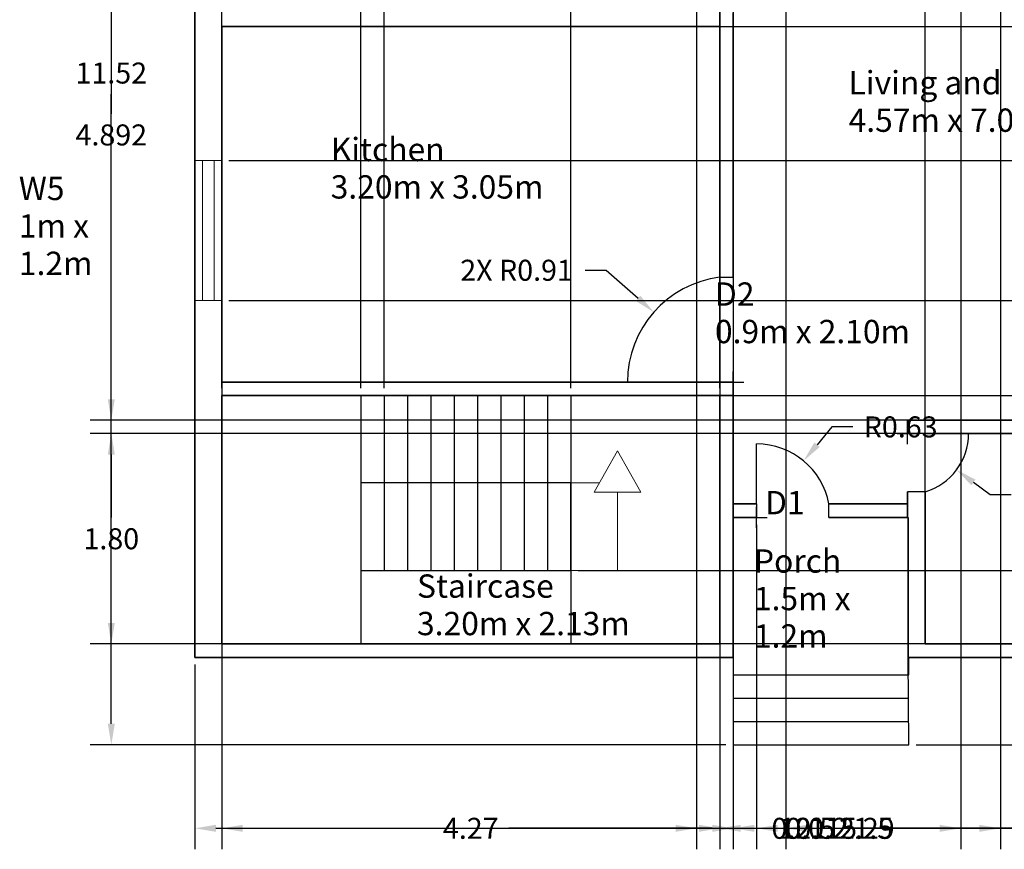
# Model space of a CAD drawing. Units: metres. Extents: x 1585.4 to 1599.4, y 2063.3 to 2076.9.
# Tile 1 of 3: x 1585.4 to 1593.9, y 2063.3 to 2070.4. Entities that reach past the tile are written whole.
import ezdxf

# ---------------------------------------------------------------- set-up
doc = ezdxf.new("R2010")
doc.units = ezdxf.units.M
for name, color, linetype, lineweight in [('A-ANNO-DIMS', 2, 'Continuous', 18), ('A-ANNO-SYMB', 7, 'Continuous', 18), ('A-ANNO-TEXT', 7, 'Continuous', 18), ('A-AREA-IDEN', 7, 'Continuous', 18), ('A-DOOR', 3, 'Continuous', 25), ('A-FLOR-STRS', 7, 'Continuous', 25), ('A-GLAZ', 4, 'Continuous', 18), ('A-WALL', 7, 'Continuous', 35)]:
    doc.layers.add(name, color=color, linetype=linetype, lineweight=lineweight)
doc.styles.get("Standard").update_dxf_attribs({"font": 'arial.ttf'})
doc.dimstyles.get("Standard").update_dxf_attribs({"dimtxt": 0.18, "dimasz": 0.18, "dimexe": 0.18, "dimexo": 0.0625, "dimgap": 0.09, "dimtad": 0, "dimtih": 1, "dimtoh": 1, "dimdec": 4, "dimzin": 0, "dimdsep": 46, "dimtxsty": 'Standard', "dimcen": 0.09, "dimadec": 0, "dimazin": 0, "dimtfac": 1, "dimtdec": 4, "dimtofl": 0, "dimtmove": 0, "dimatfit": 3, "dimfxl": 1, "dimtolj": 1, "dimtzin": 0, "dimarcsym": 0})

# ---------------------------------------------------------------- blocks, each defined once
blk = doc.blocks.new('WIN-FRAME-1200')
for p, q in [((0, 0), (0, 1.2)), ((0, 1.2), (0.23, 1.2)), ((0.23, 0), (0, 0))]:
    blk.add_line(p, q)
blk = doc.blocks.new('DOOR-900-JAMBS-SWING')
for p, q in [((0.7923, 0.9), (0.9073, 0.9)), ((0.7923, 0), (0.9073, 0))]:
    blk.add_line(p, q)
blk.add_arc((0.9073, 0), 0.9073, 97.28167, 180)
blk = doc.blocks.new('*D6')
at = {"layer": 'A-ANNO-DIMS', "color": 0, "lineweight": -2, "transparency": 16777216}
for p, q in [((1586.9308, 2064.8763), (1586.9308, 2063.2928)), ((1597.4308, 2064.8763), (1597.4308, 2063.2928)), ((1587.1108, 2063.4728), (1591.8648, 2063.4728)), ((1597.2508, 2063.4728), (1592.4968, 2063.4728))]:
    blk.add_line(p, q, dxfattribs=at)
at = {"layer": 'A-ANNO-DIMS', "color": 0, "transparency": 16777216}
for points in [[(1587.1108, 2063.5028), (1587.1108, 2063.4428), (1586.9308, 2063.4728)], [(1597.2508, 2063.5028), (1597.2508, 2063.4428), (1597.4308, 2063.4728)]]:
    blk.add_solid(points, dxfattribs=at)
at = {"layer": 'Defpoints', "color": 0, "transparency": 16777216}
for p in [(1586.9308, 2064.9388), (1597.4308, 2064.9388), (1597.4308, 2063.4728)]:
    blk.add_point(p, dxfattribs=at)
at = {"layer": 'A-ANNO-DIMS', "color": 0, "transparency": 16777216, "insert": (1592.1808, 2063.4728), "char_height": 0.18, "attachment_point": 5}
blk.add_mtext('\\A1;10.5', dxfattribs=at)
blk = doc.blocks.new('*D7')
at = {"layer": 'A-ANNO-DIMS', "color": 0, "lineweight": -2, "transparency": 16777216}
for p, q in [((1586.8683, 2075.7088), (1586.0348, 2075.7088)), ((1586.2148, 2075.5288), (1586.2148, 2070.1307)), ((1586.2148, 2064.3688), (1586.2148, 2069.7669)), ((1591.4833, 2064.1888), (1586.0348, 2064.1888))]:
    blk.add_line(p, q, dxfattribs=at)
at = {"layer": 'A-ANNO-DIMS', "color": 0, "transparency": 16777216}
for points in [[(1586.1848, 2075.5288), (1586.2448, 2075.5288), (1586.2148, 2075.7088)], [(1586.1848, 2064.3688), (1586.2448, 2064.3688), (1586.2148, 2064.1888)]]:
    blk.add_solid(points, dxfattribs=at)
at = {"layer": 'Defpoints', "color": 0, "transparency": 16777216}
for p in [(1586.2148, 2075.7088), (1586.9308, 2075.7088), (1591.5458, 2064.1888)]:
    blk.add_point(p, dxfattribs=at)
at = {"layer": 'A-ANNO-DIMS', "color": 0, "transparency": 16777216, "insert": (1586.2148, 2069.9488), "char_height": 0.18, "attachment_point": 5}
blk.add_mtext('\\A1;11.52', dxfattribs=at)
blk = doc.blocks.new('*D8')
at = {"layer": 'A-ANNO-DIMS', "color": 0, "lineweight": -2, "transparency": 16777216}
for p, q in [((1590.1533, 2067.2463), (1590.1533, 2076.6048)), ((1591.4308, 2067.2463), (1591.4308, 2076.6048)), ((1590.3333, 2076.4248), (1590.4766, 2076.4248)), ((1591.2508, 2076.4248), (1591.1076, 2076.4248))]:
    blk.add_line(p, q, dxfattribs=at)
at = {"layer": 'A-ANNO-DIMS', "color": 0, "transparency": 16777216}
for points in [[(1590.3333, 2076.4548), (1590.3333, 2076.3948), (1590.1533, 2076.4248)], [(1591.2508, 2076.4548), (1591.2508, 2076.3948), (1591.4308, 2076.4248)]]:
    blk.add_solid(points, dxfattribs=at)
at = {"layer": 'Defpoints', "color": 0, "transparency": 16777216}
for p in [(1591.4308, 2076.4248), (1590.1533, 2067.1838), (1591.4308, 2067.1838)]:
    blk.add_point(p, dxfattribs=at)
at = {"layer": 'A-ANNO-DIMS', "color": 0, "transparency": 16777216, "insert": (1590.7921, 2076.4248), "char_height": 0.18, "attachment_point": 5}
blk.add_mtext('\\A1;1.28', dxfattribs=at)
blk = doc.blocks.new('*D10')
at = {"layer": 'A-ANNO-DIMS', "color": 0, "lineweight": -2, "transparency": 16777216}
for p, q in [((1597.4933, 2064.9388), (1598.3268, 2064.9388)), ((1598.1468, 2064.7588), (1598.1468, 2064.3688)), ((1593.1124, 2064.1888), (1598.3268, 2064.1888)), ((1598.1468, 2064.1888), (1598.1468, 2064.0088)), ((1598.1468, 2064.0088), (1597.9668, 2064.0088))]:
    blk.add_line(p, q, dxfattribs=at)
at = {"layer": 'A-ANNO-DIMS', "color": 0, "transparency": 16777216}
for points in [[(1598.1168, 2064.7588), (1598.1768, 2064.7588), (1598.1468, 2064.9388)], [(1598.1168, 2064.3688), (1598.1768, 2064.3688), (1598.1468, 2064.1888)]]:
    blk.add_solid(points, dxfattribs=at)
at = {"layer": 'Defpoints', "color": 0, "transparency": 16777216}
for p in [(1597.4308, 2064.9388), (1593.0499, 2064.1888), (1598.1468, 2064.1888)]:
    blk.add_point(p, dxfattribs=at)
at = {"layer": 'A-ANNO-DIMS', "color": 0, "transparency": 16777216, "insert": (1597.6424, 2064.0088), "char_height": 0.18, "attachment_point": 5}
blk.add_mtext('\\A1;0.75', dxfattribs=at)
blk = doc.blocks.new('*D13')
at = {"layer": 'A-ANNO-DIMS', "color": 0, "lineweight": -2, "transparency": 16777216}
for p, q in [((1591.9958, 2075.4163), (1591.9958, 2063.2928)), ((1593.4958, 2075.4163), (1593.4958, 2063.2928)), ((1592.1758, 2063.4728), (1592.4998, 2063.4728)), ((1593.3158, 2063.4728), (1592.9919, 2063.4728))]:
    blk.add_line(p, q, dxfattribs=at)
at = {"layer": 'A-ANNO-DIMS', "color": 0, "transparency": 16777216}
for points in [[(1592.1758, 2063.5028), (1592.1758, 2063.4428), (1591.9958, 2063.4728)], [(1593.3158, 2063.5028), (1593.3158, 2063.4428), (1593.4958, 2063.4728)]]:
    blk.add_solid(points, dxfattribs=at)
at = {"layer": 'Defpoints', "color": 0, "transparency": 16777216}
for p in [(1591.9958, 2075.4788), (1593.4958, 2075.4788), (1593.4958, 2063.4728)]:
    blk.add_point(p, dxfattribs=at)
at = {"layer": 'A-ANNO-DIMS', "color": 0, "transparency": 16777216, "insert": (1592.7458, 2063.4728), "char_height": 0.18, "attachment_point": 5}
blk.add_mtext('\\A1;1.5', dxfattribs=at)
blk = doc.blocks.new('*D19')
at = {"layer": 'A-ANNO-DIMS', "color": 0, "lineweight": -2, "transparency": 16777216}
for p, q in [((1587.2233, 2070.3488), (1598.3268, 2070.3488)), ((1598.1468, 2070.1688), (1598.1468, 2069.9557)), ((1598.1468, 2069.3788), (1598.1468, 2069.5919)), ((1587.2233, 2069.1988), (1598.3268, 2069.1988))]:
    blk.add_line(p, q, dxfattribs=at)
at = {"layer": 'A-ANNO-DIMS', "color": 0, "transparency": 16777216}
for points in [[(1598.1168, 2070.1688), (1598.1768, 2070.1688), (1598.1468, 2070.3488)], [(1598.1168, 2069.3788), (1598.1768, 2069.3788), (1598.1468, 2069.1988)]]:
    blk.add_solid(points, dxfattribs=at)
at = {"layer": 'Defpoints', "color": 0, "transparency": 16777216}
for p in [(1587.1608, 2070.3488), (1587.1608, 2069.1988), (1598.1468, 2069.1988)]:
    blk.add_point(p, dxfattribs=at)
at = {"layer": 'A-ANNO-DIMS', "color": 0, "transparency": 16777216, "insert": (1598.1468, 2069.7738), "char_height": 0.18, "attachment_point": 5}
blk.add_mtext('\\A1;1.15', dxfattribs=at)
blk = doc.blocks.new('*D20')
at = {"layer": 'A-ANNO-DIMS', "color": 0, "lineweight": -2, "transparency": 16777216}
for p, q in [((1587.2233, 2069.1988), (1598.3268, 2069.1988)), ((1598.1468, 2069.0188), (1598.1468, 2068.7792)), ((1598.1468, 2068.1788), (1598.1468, 2068.4185)), ((1587.2233, 2067.9988), (1598.3268, 2067.9988))]:
    blk.add_line(p, q, dxfattribs=at)
at = {"layer": 'A-ANNO-DIMS', "color": 0, "transparency": 16777216}
for points in [[(1598.1168, 2069.0188), (1598.1768, 2069.0188), (1598.1468, 2069.1988)], [(1598.1168, 2068.1788), (1598.1768, 2068.1788), (1598.1468, 2067.9988)]]:
    blk.add_solid(points, dxfattribs=at)
at = {"layer": 'Defpoints', "color": 0, "transparency": 16777216}
for p in [(1587.1608, 2069.1988), (1598.1468, 2069.1988), (1587.1608, 2067.9988)]:
    blk.add_point(p, dxfattribs=at)
at = {"layer": 'A-ANNO-DIMS', "color": 0, "transparency": 16777216, "insert": (1598.1468, 2068.5988), "char_height": 0.18, "attachment_point": 5}
blk.add_mtext('\\A1;1.2', dxfattribs=at)
blk = doc.blocks.new('*D22')
at = {"layer": 'A-ANNO-DIMS', "color": 0, "lineweight": -2, "transparency": 16777216}
for p, q in [((1591.4308, 2075.4163), (1591.4308, 2063.2928)), ((1591.5458, 2075.4163), (1591.5458, 2063.2928)), ((1591.2508, 2063.4728), (1591.0708, 2063.4728)), ((1591.7258, 2063.4728), (1591.9058, 2063.4728))]:
    blk.add_line(p, q, dxfattribs=at)
at = {"layer": 'A-ANNO-DIMS', "color": 0, "transparency": 16777216}
for points in [[(1591.2508, 2063.5028), (1591.2508, 2063.4428), (1591.4308, 2063.4728)], [(1591.7258, 2063.5028), (1591.7258, 2063.4428), (1591.5458, 2063.4728)]]:
    blk.add_solid(points, dxfattribs=at)
at = {"layer": 'Defpoints', "color": 0, "transparency": 16777216}
for p in [(1591.4308, 2075.4788), (1591.5458, 2075.4788), (1591.5458, 2063.4728)]:
    blk.add_point(p, dxfattribs=at)
at = {"layer": 'A-ANNO-DIMS', "color": 0, "transparency": 16777216, "insert": (1592.3002, 2063.4728), "char_height": 0.18, "attachment_point": 5}
blk.add_mtext('\\A1;0.115', dxfattribs=at)
blk = doc.blocks.new('*D23')
at = {"layer": 'A-ANNO-DIMS', "color": 0, "lineweight": -2, "transparency": 16777216}
for p, q in [((1591.5458, 2072.9013), (1591.5458, 2063.2928)), ((1593.8358, 2072.9013), (1593.8358, 2063.2928)), ((1591.7258, 2063.4728), (1592.3653, 2063.4728)), ((1593.6558, 2063.4728), (1593.0163, 2063.4728))]:
    blk.add_line(p, q, dxfattribs=at)
at = {"layer": 'A-ANNO-DIMS', "color": 0, "transparency": 16777216}
for points in [[(1591.7258, 2063.5028), (1591.7258, 2063.4428), (1591.5458, 2063.4728)], [(1593.6558, 2063.5028), (1593.6558, 2063.4428), (1593.8358, 2063.4728)]]:
    blk.add_solid(points, dxfattribs=at)
at = {"layer": 'Defpoints', "color": 0, "transparency": 16777216}
for p in [(1591.5458, 2072.9638), (1593.8358, 2072.9638), (1593.8358, 2063.4728)]:
    blk.add_point(p, dxfattribs=at)
at = {"layer": 'A-ANNO-DIMS', "color": 0, "transparency": 16777216, "insert": (1592.6908, 2063.4728), "char_height": 0.18, "attachment_point": 5}
blk.add_mtext('\\A1;2.29', dxfattribs=at)
blk = doc.blocks.new('*D25')
at = {"layer": 'A-ANNO-DIMS', "color": 0, "lineweight": -2, "transparency": 16777216}
for p, q in [((1597.1383, 2066.8573), (1586.0348, 2066.8573)), ((1586.2148, 2066.6773), (1586.2148, 2066.1375)), ((1586.2148, 2065.2338), (1586.2148, 2065.7737)), ((1597.1383, 2065.0538), (1586.0348, 2065.0538))]:
    blk.add_line(p, q, dxfattribs=at)
at = {"layer": 'A-ANNO-DIMS', "color": 0, "transparency": 16777216}
for points in [[(1586.1848, 2066.6773), (1586.2448, 2066.6773), (1586.2148, 2066.8573)], [(1586.1848, 2065.2338), (1586.2448, 2065.2338), (1586.2148, 2065.0538)]]:
    blk.add_solid(points, dxfattribs=at)
at = {"layer": 'Defpoints', "color": 0, "transparency": 16777216}
for p in [(1586.2148, 2066.8573), (1597.2008, 2066.8573), (1597.2008, 2065.0538)]:
    blk.add_point(p, dxfattribs=at)
at = {"layer": 'A-ANNO-DIMS', "color": 0, "transparency": 16777216, "insert": (1586.2148, 2065.9556), "char_height": 0.18, "attachment_point": 5}
blk.add_mtext('\\A1;1.80', dxfattribs=at)
blk = doc.blocks.new('*D26')
at = {"layer": 'A-ANNO-DIMS', "color": 0, "lineweight": -2, "transparency": 16777216}
for p, q in [((1593.1908, 2065.1163), (1593.1908, 2076.6048)), ((1597.2008, 2065.1163), (1597.2008, 2076.6048)), ((1593.3708, 2076.4248), (1594.8858, 2076.4248)), ((1597.0208, 2076.4248), (1595.5058, 2076.4248))]:
    blk.add_line(p, q, dxfattribs=at)
at = {"layer": 'A-ANNO-DIMS', "color": 0, "transparency": 16777216}
for points in [[(1593.3708, 2076.4548), (1593.3708, 2076.3948), (1593.1908, 2076.4248)], [(1597.0208, 2076.4548), (1597.0208, 2076.3948), (1597.2008, 2076.4248)]]:
    blk.add_solid(points, dxfattribs=at)
at = {"layer": 'Defpoints', "color": 0, "transparency": 16777216}
for p in [(1597.2008, 2076.4248), (1593.1908, 2065.0538), (1597.2008, 2065.0538)]:
    blk.add_point(p, dxfattribs=at)
at = {"layer": 'A-ANNO-DIMS', "color": 0, "transparency": 16777216, "insert": (1595.1958, 2076.4248), "char_height": 0.18, "attachment_point": 5}
blk.add_mtext('\\A1;4.01', dxfattribs=at)
blk = doc.blocks.new('*D27')
at = {"layer": 'A-ANNO-DIMS', "color": 0, "lineweight": -2, "transparency": 16777216}
for p, q in [((1587.1608, 2067.2463), (1587.1608, 2076.6048)), ((1588.3533, 2067.2463), (1588.3533, 2076.6048)), ((1587.3408, 2076.4248), (1587.4416, 2076.4248)), ((1588.1733, 2076.4248), (1588.0726, 2076.4248))]:
    blk.add_line(p, q, dxfattribs=at)
at = {"layer": 'A-ANNO-DIMS', "color": 0, "transparency": 16777216}
for points in [[(1587.3408, 2076.4548), (1587.3408, 2076.3948), (1587.1608, 2076.4248)], [(1588.1733, 2076.4548), (1588.1733, 2076.3948), (1588.3533, 2076.4248)]]:
    blk.add_solid(points, dxfattribs=at)
at = {"layer": 'Defpoints', "color": 0, "transparency": 16777216}
for p in [(1588.3533, 2076.4248), (1587.1608, 2067.1838), (1588.3533, 2067.1838)]:
    blk.add_point(p, dxfattribs=at)
at = {"layer": 'A-ANNO-DIMS', "color": 0, "transparency": 16777216, "insert": (1587.7571, 2076.4248), "char_height": 0.18, "attachment_point": 5}
blk.add_mtext('\\A1;1.19', dxfattribs=at)
blk = doc.blocks.new('*D28')
at = {"layer": 'A-ANNO-DIMS', "color": 0, "lineweight": -2, "transparency": 16777216}
for p, q in [((1588.3533, 2067.2463), (1588.3533, 2076.6048)), ((1588.5533, 2067.2463), (1588.5533, 2076.6048)), ((1588.1733, 2076.4248), (1587.9933, 2076.4248)), ((1588.7333, 2076.4248), (1588.9133, 2076.4248))]:
    blk.add_line(p, q, dxfattribs=at)
at = {"layer": 'A-ANNO-DIMS', "color": 0, "transparency": 16777216}
for points in [[(1588.1733, 2076.4548), (1588.1733, 2076.3948), (1588.3533, 2076.4248)], [(1588.7333, 2076.4548), (1588.7333, 2076.3948), (1588.5533, 2076.4248)]]:
    blk.add_solid(points, dxfattribs=at)
at = {"layer": 'Defpoints', "color": 0, "transparency": 16777216}
for p in [(1588.5533, 2076.4248), (1588.3533, 2067.1838), (1588.5533, 2067.1838)]:
    blk.add_point(p, dxfattribs=at)
at = {"layer": 'A-ANNO-DIMS', "color": 0, "transparency": 16777216, "insert": (1589.1663, 2076.4248), "char_height": 0.18, "attachment_point": 5}
blk.add_mtext('\\A1;0.2', dxfattribs=at)
blk = doc.blocks.new('*D29')
at = {"layer": 'A-ANNO-DIMS', "color": 0, "lineweight": -2, "transparency": 16777216}
for p, q in [((1590.2158, 2067.1838), (1598.3268, 2067.1838)), ((1598.1468, 2067.0038), (1598.1468, 2066.6157)), ((1598.1468, 2065.8638), (1598.1468, 2066.2519)), ((1590.2158, 2065.6838), (1598.3268, 2065.6838))]:
    blk.add_line(p, q, dxfattribs=at)
at = {"layer": 'A-ANNO-DIMS', "color": 0, "transparency": 16777216}
for points in [[(1598.1168, 2067.0038), (1598.1768, 2067.0038), (1598.1468, 2067.1838)], [(1598.1168, 2065.8638), (1598.1768, 2065.8638), (1598.1468, 2065.6838)]]:
    blk.add_solid(points, dxfattribs=at)
at = {"layer": 'Defpoints', "color": 0, "transparency": 16777216}
for p in [(1590.1533, 2067.1838), (1590.1533, 2065.6838), (1598.1468, 2065.6838)]:
    blk.add_point(p, dxfattribs=at)
at = {"layer": 'A-ANNO-DIMS', "color": 0, "transparency": 16777216, "insert": (1598.1468, 2066.4338), "char_height": 0.18, "attachment_point": 5}
blk.add_mtext('\\A1;1.5', dxfattribs=at)
blk = doc.blocks.new('*D30')
at = {"layer": 'A-ANNO-DIMS', "color": 0, "lineweight": -2, "transparency": 16777216}
for p, q in [((1591.5458, 2066.0763), (1591.5458, 2063.2928)), ((1591.7458, 2066.0763), (1591.7458, 2063.2928)), ((1591.3658, 2063.4728), (1591.1858, 2063.4728)), ((1591.9258, 2063.4728), (1592.1058, 2063.4728))]:
    blk.add_line(p, q, dxfattribs=at)
at = {"layer": 'A-ANNO-DIMS', "color": 0, "transparency": 16777216}
for points in [[(1591.3658, 2063.5028), (1591.3658, 2063.4428), (1591.5458, 2063.4728)], [(1591.9258, 2063.5028), (1591.9258, 2063.4428), (1591.7458, 2063.4728)]]:
    blk.add_solid(points, dxfattribs=at)
at = {"layer": 'Defpoints', "color": 0, "transparency": 16777216}
for p in [(1591.5458, 2066.1388), (1591.7458, 2066.1388), (1591.7458, 2063.4728)]:
    blk.add_point(p, dxfattribs=at)
at = {"layer": 'A-ANNO-DIMS', "color": 0, "transparency": 16777216, "insert": (1592.3588, 2063.4728), "char_height": 0.18, "attachment_point": 5}
blk.add_mtext('\\A1;0.2', dxfattribs=at)
blk = doc.blocks.new('*D31')
at = {"layer": 'A-ANNO-DIMS', "color": 0, "lineweight": -2, "transparency": 16777216}
for p, q in [((1593.8358, 2071.8013), (1593.8358, 2063.2928)), ((1594.1508, 2071.8013), (1594.1508, 2063.2928)), ((1593.6558, 2063.4728), (1593.4758, 2063.4728)), ((1594.3308, 2063.4728), (1594.5108, 2063.4728))]:
    blk.add_line(p, q, dxfattribs=at)
at = {"layer": 'A-ANNO-DIMS', "color": 0, "transparency": 16777216}
for points in [[(1593.6558, 2063.5028), (1593.6558, 2063.4428), (1593.8358, 2063.4728)], [(1594.3308, 2063.5028), (1594.3308, 2063.4428), (1594.1508, 2063.4728)]]:
    blk.add_solid(points, dxfattribs=at)
at = {"layer": 'Defpoints', "color": 0, "transparency": 16777216}
for p in [(1593.8358, 2071.8638), (1594.1508, 2071.8638), (1594.1508, 2063.4728)]:
    blk.add_point(p, dxfattribs=at)
at = {"layer": 'A-ANNO-DIMS', "color": 0, "transparency": 16777216, "insert": (1594.9052, 2063.4728), "char_height": 0.18, "attachment_point": 5}
blk.add_mtext('\\A1;0.315', dxfattribs=at)
blk = doc.blocks.new('*D32')
at = {"layer": 'A-ANNO-DIMS', "color": 0, "lineweight": -2, "transparency": 16777216}
for p, q in [((1591.4308, 2071.9163), (1591.4308, 2063.2928)), ((1591.2308, 2071.8013), (1591.2308, 2063.2928)), ((1591.0508, 2063.4728), (1590.8708, 2063.4728)), ((1591.6108, 2063.4728), (1591.7908, 2063.4728))]:
    blk.add_line(p, q, dxfattribs=at)
at = {"layer": 'A-ANNO-DIMS', "color": 0, "transparency": 16777216}
for points in [[(1591.0508, 2063.5028), (1591.0508, 2063.4428), (1591.2308, 2063.4728)], [(1591.6108, 2063.5028), (1591.6108, 2063.4428), (1591.4308, 2063.4728)]]:
    blk.add_solid(points, dxfattribs=at)
at = {"layer": 'Defpoints', "color": 0, "transparency": 16777216}
for p in [(1591.4308, 2071.9788), (1591.2308, 2071.8638), (1591.4308, 2063.4728)]:
    blk.add_point(p, dxfattribs=at)
at = {"layer": 'A-ANNO-DIMS', "color": 0, "transparency": 16777216, "insert": (1592.0438, 2063.4728), "char_height": 0.18, "attachment_point": 5}
blk.add_mtext('\\A1;0.2', dxfattribs=at)
blk = doc.blocks.new('*D33')
at = {"layer": 'A-ANNO-DIMS', "color": 0, "lineweight": -2, "transparency": 16777216}
for p, q in [((1587.1608, 2070.2863), (1587.1608, 2063.2928)), ((1591.4308, 2070.2863), (1591.4308, 2063.2928)), ((1587.3408, 2063.4728), (1588.9684, 2063.4728)), ((1591.2508, 2063.4728), (1589.6232, 2063.4728))]:
    blk.add_line(p, q, dxfattribs=at)
at = {"layer": 'A-ANNO-DIMS', "color": 0, "transparency": 16777216}
for points in [[(1587.3408, 2063.5028), (1587.3408, 2063.4428), (1587.1608, 2063.4728)], [(1591.2508, 2063.5028), (1591.2508, 2063.4428), (1591.4308, 2063.4728)]]:
    blk.add_solid(points, dxfattribs=at)
at = {"layer": 'Defpoints', "color": 0, "transparency": 16777216}
for p in [(1587.1608, 2070.3488), (1591.4308, 2070.3488), (1591.4308, 2063.4728)]:
    blk.add_point(p, dxfattribs=at)
at = {"layer": 'A-ANNO-DIMS', "color": 0, "transparency": 16777216, "insert": (1589.2958, 2063.4728), "char_height": 0.18, "attachment_point": 5}
blk.add_mtext('\\A1;4.27', dxfattribs=at)
blk = doc.blocks.new('*D36')
at = {"layer": 'A-ANNO-DIMS', "color": 0, "lineweight": -2, "transparency": 16777216}
for p, q in [((1597.2008, 2070.4598), (1597.2008, 2063.2928)), ((1591.5458, 2070.4013), (1591.5458, 2063.2928)), ((1591.7258, 2063.4728), (1593.9789, 2063.4728)), ((1597.0208, 2063.4728), (1594.7677, 2063.4728))]:
    blk.add_line(p, q, dxfattribs=at)
at = {"layer": 'A-ANNO-DIMS', "color": 0, "transparency": 16777216}
for points in [[(1591.7258, 2063.5028), (1591.7258, 2063.4428), (1591.5458, 2063.4728)], [(1597.0208, 2063.5028), (1597.0208, 2063.4428), (1597.2008, 2063.4728)]]:
    blk.add_solid(points, dxfattribs=at)
at = {"layer": 'Defpoints', "color": 0, "transparency": 16777216}
for p in [(1597.2008, 2070.5223), (1591.5458, 2070.4638), (1597.2008, 2063.4728)]:
    blk.add_point(p, dxfattribs=at)
at = {"layer": 'A-ANNO-DIMS', "color": 0, "transparency": 16777216, "insert": (1594.3733, 2063.4728), "char_height": 0.18, "attachment_point": 5}
blk.add_mtext('\\A1;5.655', dxfattribs=at)
blk = doc.blocks.new('*D37')
at = {"layer": 'A-ANNO-DIMS', "color": 0, "lineweight": -2, "transparency": 16777216}
for p, q in [((1597.1383, 2071.8638), (1586.0348, 2071.8638)), ((1586.2148, 2071.6838), (1586.2148, 2069.6)), ((1586.2148, 2067.1523), (1586.2148, 2069.2362)), ((1597.1383, 2066.9723), (1586.0348, 2066.9723))]:
    blk.add_line(p, q, dxfattribs=at)
at = {"layer": 'A-ANNO-DIMS', "color": 0, "transparency": 16777216}
for points in [[(1586.1848, 2071.6838), (1586.2448, 2071.6838), (1586.2148, 2071.8638)], [(1586.1848, 2067.1523), (1586.2448, 2067.1523), (1586.2148, 2066.9723)]]:
    blk.add_solid(points, dxfattribs=at)
at = {"layer": 'Defpoints', "color": 0, "transparency": 16777216}
for p in [(1586.2148, 2071.8638), (1597.2008, 2071.8638), (1597.2008, 2066.9723)]:
    blk.add_point(p, dxfattribs=at)
at = {"layer": 'A-ANNO-DIMS', "color": 0, "transparency": 16777216, "insert": (1586.2148, 2069.4181), "char_height": 0.18, "attachment_point": 5}
blk.add_mtext('\\A1;4.892', dxfattribs=at)
blk = doc.blocks.new('*D38')
at = {"layer": 'A-ANNO-DIMS', "color": 0, "lineweight": -2, "transparency": 16777216}
for p, q in [((1590.276, 2068.2579), (1590.456, 2068.2579)), ((1590.456, 2068.2579), (1590.7296, 2068.0172)), ((1591.5458, 2067.2088), (1591.5458, 2067.3888)), ((1591.4558, 2067.2988), (1591.6358, 2067.2988))]:
    blk.add_line(p, q, dxfattribs=at)
at = {"layer": 'A-ANNO-DIMS', "color": 0, "transparency": 16777216}
blk.add_solid([(1590.7494, 2068.0397), (1590.7098, 2067.9947), (1590.8647, 2067.8983)], dxfattribs=at)
at = {"layer": 'Defpoints', "color": 0, "transparency": 16777216}
for p in [(1590.8647, 2067.8983), (1591.5458, 2067.2988)]:
    blk.add_point(p, dxfattribs=at)
at = {"layer": 'A-ANNO-DIMS', "color": 0, "transparency": 16777216, "insert": (1589.6886, 2068.2579), "char_height": 0.18, "attachment_point": 5}
blk.add_mtext('\\A1;2X R0.91', dxfattribs=at)
blk = doc.blocks.new('*D42')
at = {"layer": 'A-ANNO-DIMS', "color": 0, "lineweight": -2, "transparency": 16777216}
for p, q in [((1592.3907, 2066.9148), (1592.2639, 2066.7623)), ((1592.5707, 2066.9148), (1592.3907, 2066.9148)), ((1591.7458, 2066.0488), (1591.7458, 2066.2288)), ((1591.6558, 2066.1388), (1591.8358, 2066.1388))]:
    blk.add_line(p, q, dxfattribs=at)
at = {"layer": 'A-ANNO-DIMS', "color": 0, "transparency": 16777216}
blk.add_solid([(1592.2408, 2066.7814), (1592.287, 2066.7431), (1592.1488, 2066.6238)], dxfattribs=at)
at = {"layer": 'Defpoints', "color": 0, "transparency": 16777216}
for p in [(1592.1488, 2066.6238), (1591.7458, 2066.1388)]:
    blk.add_point(p, dxfattribs=at)
at = {"layer": 'A-ANNO-DIMS', "color": 0, "transparency": 16777216, "insert": (1592.9806, 2066.9148), "char_height": 0.18, "attachment_point": 5}
blk.add_mtext('\\A1;R0.63', dxfattribs=at)
blk = doc.blocks.new('*D43')
at = {"layer": 'A-ANNO-DIMS', "color": 0, "lineweight": -2, "transparency": 16777216}
for p, q in [((1593.0408, 2066.7673), (1593.0408, 2066.9473)), ((1592.9508, 2066.8573), (1593.1308, 2066.8573)), ((1593.7489, 2066.3314), (1593.6044, 2066.4388)), ((1593.9289, 2066.3314), (1593.7489, 2066.3314))]:
    blk.add_line(p, q, dxfattribs=at)
at = {"layer": 'A-ANNO-DIMS', "color": 0, "transparency": 16777216}
blk.add_solid([(1593.6223, 2066.4628), (1593.5865, 2066.4147), (1593.4599, 2066.5461)], dxfattribs=at)
at = {"layer": 'Defpoints', "color": 0, "transparency": 16777216}
for p in [(1593.0408, 2066.8573), (1593.4599, 2066.5461)]:
    blk.add_point(p, dxfattribs=at)
at = {"layer": 'A-ANNO-DIMS', "color": 0, "transparency": 16777216, "insert": (1594.4078, 2066.3314), "char_height": 0.18, "attachment_point": 5}
blk.add_mtext('\\A1;R0.522', dxfattribs=at)

msp = doc.modelspace()

# ---------------------------------------------------------------- linework, layer by layer
at = {"layer": 'A-ANNO-SYMB'}
for p, q in [((1590.5533, 2066.709), (1590.3533, 2066.356)), ((1590.7533, 2066.356), (1590.5533, 2066.709)), ((1590.5533, 2066.356), (1590.3533, 2066.356)), ((1590.3533, 2066.356), (1590.7533, 2066.356)), ((1590.3533, 2066.356), (1590.7533, 2066.356)), ((1590.5533, 2065.6838), (1590.5533, 2066.356)), ((1590.7533, 2066.356), (1590.5533, 2066.356)), ((1590.1533, 2065.6838), (1590.5533, 2065.6838))]:
    msp.add_line(p, q, dxfattribs=at)
msp.add_lwpolyline([(1590.1533, 2066.4338), (1590.3974, 2066.4338)], dxfattribs=at)
at = {"layer": 'A-DOOR'}
for p, q in [((1591.5458, 2067.2988), (1591.4308, 2067.2988)), ((1593.1908, 2066.8573), (1593.0408, 2066.8573)), ((1591.7458, 2066.2538), (1591.7458, 2066.7694)), ((1593.1908, 2066.3573), (1593.0408, 2066.3573)), ((1591.7458, 2066.2538), (1591.7458, 2066.1388)), ((1592.3658, 2066.1388), (1592.3658, 2066.2538))]:
    msp.add_line(p, q, dxfattribs=at)
for centre, radius, start, end in [((1593.0408, 2066.8573), 0.522, 286.69924, 0), ((1591.7458, 2066.1388), 0.6306, 10.50802, 90)]:
    msp.add_arc(centre, radius, start, end, dxfattribs=at)
at = {"layer": 'A-FLOR-STRS'}
for p, q in [((1588.3533, 2067.1838), (1588.3533, 2065.6838)), ((1588.5533, 2067.1838), (1588.5533, 2065.6838)), ((1588.7533, 2067.1838), (1588.7533, 2065.6838)), ((1588.9533, 2067.1838), (1588.9533, 2065.6838)), ((1589.1533, 2067.1838), (1589.1533, 2065.6838)), ((1589.3533, 2067.1838), (1589.3533, 2065.6838)), ((1589.5533, 2067.1838), (1589.5533, 2065.6838)), ((1589.7533, 2067.1838), (1589.7533, 2065.6838)), ((1589.9533, 2067.1838), (1589.9533, 2065.6838)), ((1590.1533, 2067.1838), (1590.1533, 2065.6838)), ((1590.1533, 2066.4338), (1588.3533, 2066.4338)), ((1590.1533, 2065.6838), (1590.1533, 2066.4338)), ((1588.3533, 2065.6838), (1590.1533, 2065.6838)), ((1588.3533, 2065.6838), (1588.3533, 2065.0538)), ((1590.1533, 2065.6838), (1590.1533, 2065.0538)), ((1591.5458, 2064.9388), (1591.5458, 2064.7888)), ((1593.0499, 2064.1888), (1593.0458, 2064.9388)), ((1593.0499, 2064.7888), (1593.0499, 2064.9388)), ((1591.5458, 2064.7888), (1593.0499, 2064.7888)), ((1591.5458, 2064.7888), (1591.5458, 2064.1888)), ((1591.5458, 2064.5888), (1593.0499, 2064.5888)), ((1591.5458, 2064.3888), (1593.0499, 2064.3888)), ((1591.5458, 2064.1888), (1593.0499, 2064.1888)), ((1591.5458, 2064.1888), (1593.0499, 2064.1888))]:
    msp.add_line(p, q, dxfattribs=at)
at = {"layer": 'A-GLAZ'}
for p, q in [((1586.9958, 2069.1988), (1586.9958, 2067.9988)), ((1587.0958, 2069.1988), (1587.0958, 2067.9988))]:
    msp.add_line(p, q, dxfattribs=at)
at = {"layer": 'A-WALL'}
for p, q in [((1591.5458, 2070.4638), (1591.5458, 2068.1988)), ((1589.5608, 2070.3488), (1587.1608, 2070.3488)), ((1587.1608, 2070.3488), (1587.1608, 2067.2988)), ((1591.4308, 2070.3488), (1589.5608, 2070.3488)), ((1591.4308, 2068.1988), (1591.4308, 2070.3488)), ((1587.1608, 2067.2988), (1587.1608, 2067.9988)), ((1587.1608, 2067.2988), (1591.4308, 2067.2988)), ((1591.5458, 2067.2988), (1591.5458, 2067.1838)), ((1591.5458, 2067.1838), (1587.1608, 2067.1838)), ((1587.1608, 2067.1838), (1587.1608, 2065.0538)), ((1591.4308, 2065.0538), (1591.4308, 2067.1838)), ((1591.4308, 2067.1838), (1591.5458, 2067.1838)), ((1591.5458, 2067.1838), (1591.5458, 2065.0538)), ((1597.2008, 2066.9723), (1593.0408, 2066.9723)), ((1593.0408, 2066.9723), (1593.0408, 2066.8573)), ((1593.1908, 2066.8573), (1597.2008, 2066.8573)), ((1593.0408, 2066.3573), (1593.0408, 2066.1388)), ((1593.1908, 2065.0538), (1593.1908, 2066.3573)), ((1591.5458, 2066.1388), (1591.5458, 2066.2538)), ((1591.5458, 2066.2538), (1591.7458, 2066.2538)), ((1591.5458, 2066.2538), (1591.7458, 2066.2538)), ((1592.3658, 2066.2538), (1593.0408, 2066.2538)), ((1591.5458, 2064.9388), (1591.5458, 2066.1388)), ((1591.5458, 2064.9388), (1591.5458, 2066.1388)), ((1591.5458, 2066.1388), (1591.7458, 2066.1388)), ((1592.3658, 2066.1388), (1593.0458, 2066.1388)), ((1593.0458, 2066.1388), (1593.0458, 2064.9388)), ((1587.1608, 2065.0538), (1591.4308, 2065.0538)), ((1591.5458, 2065.0538), (1591.5458, 2064.9388)), ((1597.2008, 2065.0538), (1593.1908, 2065.0538)), ((1591.5458, 2064.9388), (1586.9308, 2064.9388)), ((1593.0458, 2064.9388), (1597.2008, 2064.9388))]:
    msp.add_line(p, q, dxfattribs=at)
msp.add_lwpolyline([(1597.4308, 2064.9388), (1597.4308, 2075.7088), (1586.9308, 2075.7088), (1586.9308, 2064.9388)], dxfattribs=at)

# ---------------------------------------------------------------- block references
at = {"layer": 'A-DOOR'}
msp.add_blockref('DOOR-900-JAMBS-SWING', (1590.6385, 2067.2988), dxfattribs=at)
at = {"layer": 'A-GLAZ'}
msp.add_blockref('WIN-FRAME-1200', (1586.9308, 2067.9988), dxfattribs=at)

# ---------------------------------------------------------------- texts
at = {"layer": 'A-ANNO-TEXT'}
for s, p in [('W5', (1585.4224, 2068.8598)), ('1m x ', (1585.4224, 2068.5385)), ('1.2m', (1585.4224, 2068.2172)), ('D2', (1591.3888, 2067.9537)), ('0.9m x 2.10m', (1591.3888, 2067.6324)), ('D1', (1591.8183, 2066.1652))]:
    msp.add_text(s, height=0.2, dxfattribs=at).set_placement(p)
at = {"layer": 'A-AREA-IDEN'}
for s, p in [('Living and Dining', (1592.5343, 2069.7659)), ('4.57m x 7.01m', (1592.5343, 2069.4447)), ('Kitchen', (1588.0953, 2069.1936)), ('3.20m x 3.05m', (1588.0953, 2068.8724)), ('Porch', (1591.7229, 2065.6645)), ('Staircase', (1588.8352, 2065.4499)), ('1.5m x ', (1591.7229, 2065.3432)), ('3.20m x 2.13m', (1588.8352, 2065.1286)), ('1.2m', (1591.7229, 2065.0219))]:
    msp.add_text(s, height=0.2, dxfattribs=at).set_placement(p)

# ---------------------------------------------------------------- dimensions: what is measured, and where the dimension line sits
at = {"layer": 'A-ANNO-DIMS'}
for base, p1, p2, override, picture, middle in [((1588.3533, 2076.4248), (1587.1608, 2067.1838), (1588.3533, 2067.1838), {"dimdec": 2, "dimlfac": 1, "dimrnd": 0, "dimzin": 0, "dimdsep": 46, "dimlunit": 2}, '*D27', (1587.7571, 2076.4248)), ((1588.5533, 2076.4248), (1588.3533, 2067.1838), (1588.5533, 2067.1838), {"dimdec": 1, "dimlfac": 1, "dimrnd": 0, "dimzin": 0, "dimdsep": 46, "dimlunit": 2}, '*D28', (1589.1663, 2076.4248)), ((1591.4308, 2076.4248), (1590.1533, 2067.1838), (1591.4308, 2067.1838), {"dimdec": 2, "dimlfac": 1, "dimrnd": 0, "dimzin": 0, "dimdsep": 46, "dimlunit": 2}, '*D8', (1590.7921, 2076.4248)), ((1597.2008, 2076.4248), (1593.1908, 2065.0538), (1597.2008, 2065.0538), {"dimdec": 2, "dimlfac": 1, "dimrnd": 0, "dimzin": 0, "dimdsep": 46, "dimlunit": 2}, '*D26', (1595.1958, 2076.4248)), ((1591.5458, 2063.4728), (1591.4308, 2075.4788), (1591.5458, 2075.4788), {"dimdec": 3, "dimlfac": 1, "dimrnd": 0, "dimzin": 0, "dimdsep": 46, "dimlunit": 2}, '*D22', (1592.3002, 2063.4728)), ((1593.4958, 2063.4728), (1591.9958, 2075.4788), (1593.4958, 2075.4788), {"dimdec": 1, "dimlfac": 1, "dimrnd": 0, "dimzin": 0, "dimdsep": 46, "dimlunit": 2}, '*D13', (1592.7458, 2063.4728)), ((1593.8358, 2063.4728), (1591.5458, 2072.9638), (1593.8358, 2072.9638), {"dimdec": 2, "dimlfac": 1, "dimrnd": 0, "dimzin": 0, "dimdsep": 46, "dimlunit": 2}, '*D23', (1592.6908, 2063.4728)), ((1591.4308, 2063.4728), (1591.2308, 2071.8638), (1591.4308, 2071.9788), {"dimdec": 1, "dimlfac": 1, "dimrnd": 0, "dimzin": 0, "dimdsep": 46, "dimlunit": 2}, '*D32', (1592.0438, 2063.4728)), ((1594.1508, 2063.4728), (1593.8358, 2071.8638), (1594.1508, 2071.8638), {"dimdec": 3, "dimlfac": 1, "dimrnd": 0, "dimzin": 0, "dimdsep": 46, "dimlunit": 2}, '*D31', (1594.9052, 2063.4728)), ((1597.2008, 2063.4728), (1591.5458, 2070.4638), (1597.2008, 2070.5223), {"dimdec": 3, "dimlfac": 1, "dimrnd": 0, "dimzin": 0, "dimdsep": 46, "dimlunit": 2}, '*D36', (1594.3733, 2063.4728)), ((1591.4308, 2063.4728), (1587.1608, 2070.3488), (1591.4308, 2070.3488), {"dimdec": 2, "dimlfac": 1, "dimrnd": 0, "dimzin": 0, "dimdsep": 46, "dimlunit": 2}, '*D33', (1589.2958, 2063.4728)), ((1591.7458, 2063.4728), (1591.5458, 2066.1388), (1591.7458, 2066.1388), {"dimdec": 1, "dimlfac": 1, "dimrnd": 0, "dimzin": 0, "dimdsep": 46, "dimlunit": 2}, '*D30', (1592.3588, 2063.4728)), ((1597.4308, 2063.4728), (1586.9308, 2064.9388), (1597.4308, 2064.9388), {"dimdec": 1, "dimlfac": 1, "dimrnd": 0, "dimzin": 0, "dimdsep": 46, "dimlunit": 2}, '*D6', (1592.1808, 2063.4728))]:
    dim = msp.add_linear_dim(base=base, p1=p1, p2=p2, dimstyle='Standard', override=override, dxfattribs=at)
    dim.commit()
    dim.dimension.update_dxf_attribs({"geometry": picture, "text_midpoint": middle})
for base, p1, p2, override, picture, middle in [((1586.2148, 2075.7088), (1591.5458, 2064.1888), (1586.9308, 2075.7088), {"dimdec": 2, "dimlfac": 1, "dimrnd": 0, "dimzin": 0, "dimdsep": 46, "dimlunit": 2}, '*D7', (1586.2148, 2069.9488)), ((1586.21482, 2071.86384), (1597.20082, 2066.97232), (1597.20082, 2071.86384), {"dimdec": 3, "dimlfac": 1, "dimrnd": 0, "dimzin": 0, "dimdsep": 46, "dimlunit": 2}, '*D37', (1586.21482, 2069.41808)), ((1598.1468, 2069.1988), (1587.1608, 2070.3488), (1587.1608, 2069.1988), {"dimdec": 2, "dimlfac": 1, "dimrnd": 0, "dimzin": 0, "dimdsep": 46, "dimlunit": 2}, '*D19', (1598.1468, 2069.7738)), ((1598.1468, 2069.1988), (1587.1608, 2067.9988), (1587.1608, 2069.1988), {"dimdec": 1, "dimlfac": 1, "dimrnd": 0, "dimzin": 0, "dimdsep": 46, "dimlunit": 2}, '*D20', (1598.1468, 2068.5988)), ((1598.1468, 2065.6838), (1590.1533, 2067.1838), (1590.1533, 2065.6838), {"dimdec": 1, "dimlfac": 1, "dimrnd": 0, "dimzin": 0, "dimdsep": 46, "dimlunit": 2}, '*D29', (1598.1468, 2066.4338)), ((1586.2148, 2066.8573), (1597.2008, 2065.0538), (1597.2008, 2066.8573), {"dimdec": 2, "dimlfac": 1, "dimrnd": 0, "dimzin": 0, "dimdsep": 46, "dimlunit": 2}, '*D25', (1586.2148, 2065.9556)), ((1598.1468, 2064.1888), (1597.4308, 2064.9388), (1593.0499, 2064.1888), {"dimdec": 2, "dimlfac": 1, "dimrnd": 0, "dimzin": 0, "dimdsep": 46, "dimlunit": 2}, '*D10', (1597.6424, 2064.0088))]:
    dim = msp.add_linear_dim(base=base, p1=p1, p2=p2, angle=90, dimstyle='Standard', override=override, dxfattribs=at)
    dim.commit()
    dim.dimension.update_dxf_attribs({"geometry": picture, "text_midpoint": middle})
dim = msp.add_radius_dim(center=(1591.5458, 2067.2988), mpoint=(1590.8647, 2067.8983), text='2X <>', dimstyle='Standard', override={"dimdec": 2, "dimlfac": 1, "dimrnd": 0, "dimzin": 0, "dimdsep": 46, "dimlunit": 2}, dxfattribs=at)
dim.commit()
dim.dimension.update_dxf_attribs({"geometry": '*D38', "text_midpoint": (1589.6886, 2068.2579), "dimtype": 164})
dim = msp.add_radius_dim(center=(1591.7458, 2066.1388), mpoint=(1592.1488, 2066.6238), dimstyle='Standard', override={"dimdec": 2, "dimlfac": 1, "dimrnd": 0, "dimzin": 0, "dimdsep": 46, "dimlunit": 2}, dxfattribs=at)
dim.commit()
dim.dimension.update_dxf_attribs({"geometry": '*D42', "text_midpoint": (1592.9806, 2066.9148), "dimtype": 164})
dim = msp.add_radius_dim(center=(1593.0408, 2066.8573), mpoint=(1593.4599, 2066.5461), dimstyle='Standard', override={"dimdec": 3, "dimlfac": 1, "dimrnd": 0, "dimzin": 0, "dimdsep": 46, "dimlunit": 2}, dxfattribs=at)
dim.commit()
dim.dimension.update_dxf_attribs({"geometry": '*D43', "text_midpoint": (1594.4078, 2066.3314)})

doc.saveas('drawing.dxf')
